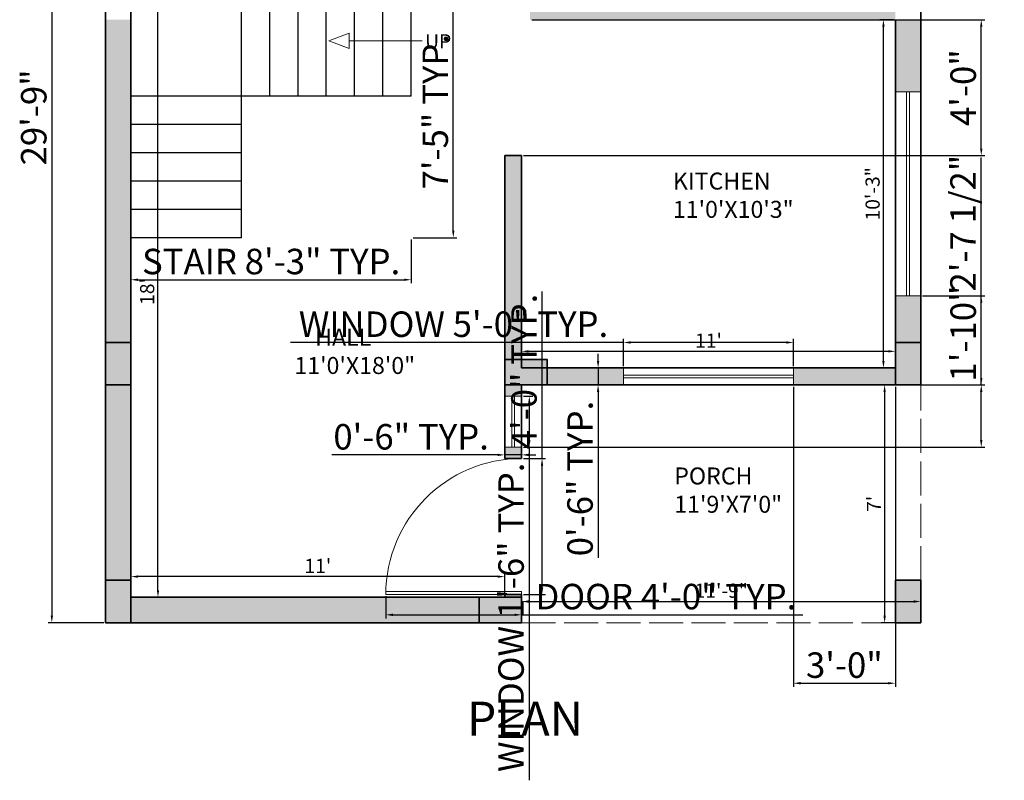
# Model space of a CAD drawing. Units: inches. Extents: x 3148 to 3962, y 1142 to 1671.
# Tile 8 of 9: x 3585 to 3933, y 1142 to 1411. Entities that reach past the tile are written whole.
import ezdxf

# ---------------------------------------------------------------- set-up
doc = ezdxf.new("R2010")
doc.units = ezdxf.units.IN
doc.linetypes.add('ACAD_ISO02W100', pattern=[15, 12, -3])
for name, color, linetype, lineweight in [('A-ANNO-DIMS', 2, 'Continuous', 18), ('A-ANNO-SYMB', 7, 'Continuous', 18), ('A-ANNO-TEXT', 7, 'Continuous', 25), ('A-AREA-IDEN', 7, 'Continuous', 18), ('A-COLS', 1, 'Continuous', 35), ('A-DOOR', 3, 'Continuous', 18), ('A-FLOR-STRS', 7, 'Continuous', 25), ('A-GLAZ', 4, 'Continuous', 18), ('A-ROOF-OVHD', 7, 'ACAD_ISO02W100', 18), ('A-WALL', 7, 'Continuous', 35)]:
    doc.layers.add(name, color=color, linetype=linetype, lineweight=lineweight)
doc.layers.add('A-WALL-PATT', color=252, linetype='Continuous', lineweight=13, true_color=0x939598)
doc.styles.get("Standard").update_dxf_attribs({"font": 'arial.ttf'})
doc.dimstyles.new('ISO-25', dxfattribs={"dimtxt": 9, "dimasz": 2.5, "dimexe": 1.25, "dimexo": 0.625, "dimtad": 1, "dimdec": 1, "dimlunit": 3, "dimtxsty": 'Standard', "dimcen": 2.5, "dimadec": 0, "dimazin": 0, "dimtfac": 1, "dimtdec": 1, "dimtmove": 0, "dimatfit": 3, "dimfxl": 1, "dimarcsym": 0})

# ---------------------------------------------------------------- blocks, each defined once
blk = doc.blocks.new('*D45')
at = {"layer": 'A-ANNO-DIMS', "color": 0, "lineweight": -2, "transparency": 16777216}
for p, q in [((3614.71, 1554.8), (3595.12, 1554.8)), ((3596.37, 1552.3), (3596.37, 1200.3)), ((3614.71, 1197.8), (3595.12, 1197.8))]:
    blk.add_line(p, q, dxfattribs=at)
at = {"layer": 'A-ANNO-DIMS', "color": 0, "transparency": 16777216}
for points in [[(3595.95, 1552.3), (3596.78, 1552.3), (3596.37, 1554.8)], [(3595.95, 1200.3), (3596.78, 1200.3), (3596.37, 1197.8)]]:
    blk.add_solid(points, dxfattribs=at)
at = {"layer": 'Defpoints', "color": 0, "transparency": 16777216}
for p in [(3615.33, 1554.8), (3596.37, 1197.8), (3615.33, 1197.8)]:
    blk.add_point(p, dxfattribs=at)
at = {"layer": 'A-ANNO-DIMS', "color": 0, "transparency": 16777216, "insert": (3591.15, 1376.3), "char_height": 9, "attachment_point": 5, "rotation": 90}
blk.add_mtext('29\'-9"', dxfattribs=at)
blk = doc.blocks.new('*D46')
at = {"layer": 'A-ANNO-DIMS', "color": 0, "lineweight": -2, "transparency": 16777216}
for p, q in [((3624.96, 1422.8), (3635.11, 1422.8)), ((3633.86, 1209.3), (3633.86, 1420.3)), ((3624.96, 1206.8), (3635.11, 1206.8))]:
    blk.add_line(p, q, dxfattribs=at)
at = {"layer": 'A-ANNO-DIMS', "color": 0, "transparency": 16777216}
for points in [[(3633.45, 1420.3), (3634.28, 1420.3), (3633.86, 1422.8)], [(3633.45, 1209.3), (3634.28, 1209.3), (3633.86, 1206.8)]]:
    blk.add_solid(points, dxfattribs=at)
at = {"layer": 'Defpoints', "color": 0, "transparency": 16777216}
for p in [(3624.33, 1422.8), (3633.86, 1422.8), (3624.33, 1206.8)]:
    blk.add_point(p, dxfattribs=at)
at = {"layer": 'A-ANNO-DIMS', "color": 0, "transparency": 16777216, "insert": (3630.69, 1314.8), "char_height": 5, "attachment_point": 5, "rotation": 90}
blk.add_mtext("18'", dxfattribs=at)
blk = doc.blocks.new('*D47')
at = {"layer": 'A-ANNO-DIMS', "color": 0, "lineweight": -2, "transparency": 16777216}
for p, q in [((3624.33, 1207.42), (3624.33, 1215.36)), ((3753.83, 1214.11), (3626.83, 1214.11)), ((3756.33, 1207.42), (3756.33, 1215.36))]:
    blk.add_line(p, q, dxfattribs=at)
at = {"layer": 'A-ANNO-DIMS', "color": 0, "transparency": 16777216}
for points in [[(3626.83, 1214.53), (3626.83, 1213.69), (3624.33, 1214.11)], [(3753.83, 1214.53), (3753.83, 1213.69), (3756.33, 1214.11)]]:
    blk.add_solid(points, dxfattribs=at)
at = {"layer": 'Defpoints', "color": 0, "transparency": 16777216}
for p in [(3624.33, 1214.11), (3624.33, 1206.8), (3756.33, 1206.8)]:
    blk.add_point(p, dxfattribs=at)
at = {"layer": 'A-ANNO-DIMS', "color": 0, "transparency": 16777216, "insert": (3690.33, 1217.24), "char_height": 5, "attachment_point": 5}
blk.add_mtext("11'", dxfattribs=at)
blk = doc.blocks.new('*D48')
at = {"layer": 'A-ANNO-DIMS', "color": 0, "lineweight": -2, "transparency": 16777216}
for p, q in [((3762.33, 1198.42), (3762.33, 1206.55)), ((3764.83, 1205.3), (3900.83, 1205.3)), ((3903.33, 1198.42), (3903.33, 1206.55))]:
    blk.add_line(p, q, dxfattribs=at)
at = {"layer": 'A-ANNO-DIMS', "color": 0, "transparency": 16777216}
for points in [[(3764.83, 1205.72), (3764.83, 1204.88), (3762.33, 1205.3)], [(3900.83, 1205.72), (3900.83, 1204.88), (3903.33, 1205.3)]]:
    blk.add_solid(points, dxfattribs=at)
at = {"layer": 'Defpoints', "color": 0, "transparency": 16777216}
for p in [(3903.33, 1205.3), (3762.33, 1197.8), (3903.33, 1197.8)]:
    blk.add_point(p, dxfattribs=at)
at = {"layer": 'A-ANNO-DIMS', "color": 0, "transparency": 16777216, "insert": (3832.83, 1208.48), "char_height": 5, "attachment_point": 5}
blk.add_mtext('11\'-9"', dxfattribs=at)
blk = doc.blocks.new('*D49')
at = {"layer": 'A-ANNO-DIMS', "color": 0, "lineweight": -2, "transparency": 16777216}
for p, q in [((3902.71, 1281.8), (3889.3, 1281.8)), ((3890.55, 1279.3), (3890.55, 1200.3)), ((3902.71, 1197.8), (3889.3, 1197.8))]:
    blk.add_line(p, q, dxfattribs=at)
at = {"layer": 'A-ANNO-DIMS', "color": 0, "transparency": 16777216}
for points in [[(3890.13, 1279.3), (3890.96, 1279.3), (3890.55, 1281.8)], [(3890.13, 1200.3), (3890.96, 1200.3), (3890.55, 1197.8)]]:
    blk.add_solid(points, dxfattribs=at)
at = {"layer": 'Defpoints', "color": 0, "transparency": 16777216}
for p in [(3903.33, 1281.8), (3890.55, 1197.8), (3903.33, 1197.8)]:
    blk.add_point(p, dxfattribs=at)
at = {"layer": 'A-ANNO-DIMS', "color": 0, "transparency": 16777216, "insert": (3887.42, 1239.8), "char_height": 5, "attachment_point": 5, "rotation": 90}
blk.add_mtext("7'", dxfattribs=at)
blk = doc.blocks.new('*D50')
at = {"layer": 'A-ANNO-DIMS', "color": 0, "lineweight": -2, "transparency": 16777216}
for p, q in [((3762.33, 1291.42), (3762.33, 1294.93)), ((3894.33, 1291.42), (3894.33, 1294.93)), ((3764.83, 1293.68), (3891.83, 1293.68))]:
    blk.add_line(p, q, dxfattribs=at)
at = {"layer": 'A-ANNO-DIMS', "color": 0, "transparency": 16777216}
for points in [[(3764.83, 1294.09), (3764.83, 1293.26), (3762.33, 1293.68)], [(3891.83, 1294.09), (3891.83, 1293.26), (3894.33, 1293.68)]]:
    blk.add_solid(points, dxfattribs=at)
at = {"layer": 'Defpoints', "color": 0, "transparency": 16777216}
for p in [(3762.33, 1290.8), (3894.33, 1293.68), (3894.33, 1290.8)]:
    blk.add_point(p, dxfattribs=at)
at = {"layer": 'A-ANNO-DIMS', "color": 0, "transparency": 16777216, "insert": (3828.33, 1296.81), "char_height": 5, "attachment_point": 5}
blk.add_mtext("11'", dxfattribs=at)
blk = doc.blocks.new('*D51')
at = {"layer": 'A-ANNO-DIMS', "color": 0, "lineweight": -2, "transparency": 16777216}
for p, q in [((3893.71, 1410.8), (3888.88, 1410.8)), ((3890.13, 1290.3), (3890.13, 1408.3)), ((3893.71, 1287.8), (3888.88, 1287.8))]:
    blk.add_line(p, q, dxfattribs=at)
at = {"layer": 'A-ANNO-DIMS', "color": 0, "transparency": 16777216}
for points in [[(3889.71, 1408.3), (3890.55, 1408.3), (3890.13, 1410.8)], [(3889.71, 1290.3), (3890.55, 1290.3), (3890.13, 1287.8)]]:
    blk.add_solid(points, dxfattribs=at)
at = {"layer": 'Defpoints', "color": 0, "transparency": 16777216}
for p in [(3890.13, 1410.8), (3894.33, 1410.8), (3894.33, 1287.8)]:
    blk.add_point(p, dxfattribs=at)
at = {"layer": 'A-ANNO-DIMS', "color": 0, "transparency": 16777216, "insert": (3886.95, 1349.3), "char_height": 5, "attachment_point": 5, "rotation": 90}
blk.add_mtext('10\'-3"', dxfattribs=at)
blk = doc.blocks.new('DOOR-SWING-48')
for p, q in [((-48, 0), (0, 0)), ((-47.99, 1), (0, 1)), ((0, 0), (0, 1))]:
    blk.add_line(p, q)
blk.add_arc((0, 0), 48, 90, 180)
blk = doc.blocks.new('WIN-18')
for p, q in [((0, 18), (6, 18)), ((2.5, 0), (2.5, 18)), ((3.5, 0), (3.5, 18)), ((0, 0), (6, 0))]:
    blk.add_line(p, q)
blk = doc.blocks.new('WIN-60')
for p, q in [((0, 0), (0, 6)), ((60, 3.5), (0, 3.5)), ((60, 0), (60, 6)), ((60, 2.5), (0, 2.5))]:
    blk.add_line(p, q)
blk = doc.blocks.new('WIN-72')
for p, q in [((0, 72), (9, 72)), ((4, 72), (4, 0)), ((5, 72), (5, 0)), ((0, 0), (9, 0))]:
    blk.add_line(p, q)
blk = doc.blocks.new('STAIR-QUARTER-TURN')
for p, q in [((39, 0), (39, 89)), ((49, 50), (49, 89)), ((59, 50), (59, 89)), ((69, 50), (69, 89)), ((79, 50), (79, 89)), ((89, 50), (89, 89)), ((99, 50), (99, 89)), ((99, 50), (0, 50)), ((39, 40), (0, 40)), ((39, 30), (0, 30)), ((39, 20), (0, 20)), ((39, 10), (0, 10)), ((39, 0), (0, 0))]:
    blk.add_line(p, q)
blk = doc.blocks.new('COL-9X15')
h = blk.add_hatch(color=256)
h.dxf.hatch_style = 1
h.paths.add_polyline_path([(9, 15), (0, 15), (0, 0), (9, 0)])
blk.add_lwpolyline([(9, 0), (9, 15), (0, 15), (0, 0)], close=True)
blk = doc.blocks.new('STAIR-UP-ARROW')
blk.add_line((32.89, 2.71), (7.09, 2.71))
blk.add_lwpolyline([(0, 2.71), (7.09, 0), (7.09, 5.42)], close=True)
blk.add_text('UP', height=5).set_placement((33.98, 0.05))
blk = doc.blocks.new('*D76')
at = {"layer": 'A-ANNO-DIMS', "color": 0, "lineweight": -2, "transparency": 16777216}
for p, q in [((3762.96, 1277.8), (3766.28, 1277.8)), ((3765.03, 1275.3), (3765.03, 1262.3)), ((3762.96, 1259.8), (3766.28, 1259.8)), ((3765.03, 1259.8), (3765.03, 1142.16))]:
    blk.add_line(p, q, dxfattribs=at)
at = {"layer": 'A-ANNO-DIMS', "color": 0, "transparency": 16777216}
for points in [[(3764.61, 1275.3), (3765.45, 1275.3), (3765.03, 1277.8)], [(3764.61, 1262.3), (3765.45, 1262.3), (3765.03, 1259.8)]]:
    blk.add_solid(points, dxfattribs=at)
at = {"layer": 'Defpoints', "color": 0, "transparency": 16777216}
for p in [(3762.33, 1277.8), (3762.33, 1259.8), (3765.03, 1259.8)]:
    blk.add_point(p, dxfattribs=at)
at = {"layer": 'A-ANNO-DIMS', "color": 0, "transparency": 16777216, "insert": (3759.75, 1199.73), "char_height": 9, "attachment_point": 5, "rotation": 90}
blk.add_mtext('WINDOW 1\'-6" TYP.', dxfattribs=at)
blk = doc.blocks.new('*D77')
at = {"layer": 'A-ANNO-DIMS', "color": 0, "lineweight": -2, "transparency": 16777216}
for p, q in [((3756.33, 1259.17), (3756.33, 1255.85)), ((3762.33, 1259.17), (3762.33, 1255.85)), ((3753.83, 1257.1), (3695.22, 1257.1)), ((3762.33, 1257.1), (3756.33, 1257.1)), ((3764.83, 1257.1), (3767.33, 1257.1))]:
    blk.add_line(p, q, dxfattribs=at)
at = {"layer": 'A-ANNO-DIMS', "color": 0, "transparency": 16777216}
for points in [[(3753.83, 1257.52), (3753.83, 1256.68), (3756.33, 1257.1)], [(3764.83, 1257.52), (3764.83, 1256.68), (3762.33, 1257.1)]]:
    blk.add_solid(points, dxfattribs=at)
at = {"layer": 'Defpoints', "color": 0, "transparency": 16777216}
for p in [(3756.33, 1259.8), (3762.33, 1259.8), (3756.33, 1257.1)]:
    blk.add_point(p, dxfattribs=at)
at = {"layer": 'A-ANNO-DIMS', "color": 0, "transparency": 16777216, "insert": (3723.28, 1262.32), "char_height": 9, "attachment_point": 5}
blk.add_mtext('0\'-6" TYP.', dxfattribs=at)
blk = doc.blocks.new('*D78')
at = {"layer": 'A-ANNO-DIMS', "color": 0, "lineweight": -2, "transparency": 16777216}
for p, q in [((3798.33, 1288.42), (3798.33, 1298.05)), ((3858.33, 1288.42), (3858.33, 1298.05)), ((3798.33, 1296.8), (3680.69, 1296.8)), ((3855.83, 1296.8), (3800.83, 1296.8))]:
    blk.add_line(p, q, dxfattribs=at)
at = {"layer": 'A-ANNO-DIMS', "color": 0, "transparency": 16777216}
for points in [[(3800.83, 1297.22), (3800.83, 1296.38), (3798.33, 1296.8)], [(3855.83, 1297.22), (3855.83, 1296.38), (3858.33, 1296.8)]]:
    blk.add_solid(points, dxfattribs=at)
at = {"layer": 'Defpoints', "color": 0, "transparency": 16777216}
for p in [(3798.33, 1296.8), (3798.33, 1287.8), (3858.33, 1287.8)]:
    blk.add_point(p, dxfattribs=at)
at = {"layer": 'A-ANNO-DIMS', "color": 0, "transparency": 16777216, "insert": (3738.26, 1302.08), "char_height": 9, "attachment_point": 5}
blk.add_mtext('WINDOW 5\'-0" TYP.', dxfattribs=at)
blk = doc.blocks.new('*D79')
at = {"layer": 'A-ANNO-DIMS', "color": 0, "lineweight": -2, "transparency": 16777216}
for p, q in [((3789.33, 1290.3), (3789.33, 1292.8)), ((3797.71, 1287.8), (3788.08, 1287.8)), ((3789.33, 1287.8), (3789.33, 1281.8)), ((3797.71, 1281.8), (3788.08, 1281.8)), ((3789.33, 1279.3), (3789.33, 1220.69))]:
    blk.add_line(p, q, dxfattribs=at)
at = {"layer": 'A-ANNO-DIMS', "color": 0, "transparency": 16777216}
for points in [[(3788.91, 1290.3), (3789.75, 1290.3), (3789.33, 1287.8)], [(3788.91, 1279.3), (3789.75, 1279.3), (3789.33, 1281.8)]]:
    blk.add_solid(points, dxfattribs=at)
at = {"layer": 'Defpoints', "color": 0, "transparency": 16777216}
for p in [(3798.33, 1287.8), (3789.33, 1281.8), (3798.33, 1281.8)]:
    blk.add_point(p, dxfattribs=at)
at = {"layer": 'A-ANNO-DIMS', "color": 0, "transparency": 16777216, "insert": (3784.11, 1248.74), "char_height": 9, "attachment_point": 5, "rotation": 90}
blk.add_mtext('0\'-6" TYP.', dxfattribs=at)
blk = doc.blocks.new('*D84')
at = {"layer": 'A-ANNO-DIMS', "color": 0, "lineweight": -2, "transparency": 16777216}
for p, q in [((3714.33, 1207.17), (3714.33, 1199.35)), ((3762.33, 1207.17), (3762.33, 1199.35)), ((3716.83, 1200.6), (3759.83, 1200.6)), ((3762.33, 1200.6), (3861.7, 1200.6))]:
    blk.add_line(p, q, dxfattribs=at)
at = {"layer": 'A-ANNO-DIMS', "color": 0, "transparency": 16777216}
for points in [[(3716.83, 1201.02), (3716.83, 1200.18), (3714.33, 1200.6)], [(3759.83, 1201.02), (3759.83, 1200.18), (3762.33, 1200.6)]]:
    blk.add_solid(points, dxfattribs=at)
at = {"layer": 'Defpoints', "color": 0, "transparency": 16777216}
for p in [(3714.33, 1207.8), (3762.33, 1207.8), (3762.33, 1200.6)]:
    blk.add_point(p, dxfattribs=at)
at = {"layer": 'A-ANNO-DIMS', "color": 0, "transparency": 16777216, "insert": (3813.27, 1205.88), "char_height": 9, "attachment_point": 5}
blk.add_mtext('DOOR 4\'-0" TYP.', dxfattribs=at)
blk = doc.blocks.new('*D85')
at = {"layer": 'A-ANNO-DIMS', "color": 0, "lineweight": -2, "transparency": 16777216}
for p, q in [((3769.53, 1255.8), (3769.53, 1314.77)), ((3762.96, 1255.8), (3770.78, 1255.8)), ((3769.53, 1210.3), (3769.53, 1253.3)), ((3762.96, 1207.8), (3770.78, 1207.8))]:
    blk.add_line(p, q, dxfattribs=at)
at = {"layer": 'A-ANNO-DIMS', "color": 0, "transparency": 16777216}
for points in [[(3769.11, 1253.3), (3769.95, 1253.3), (3769.53, 1255.8)], [(3769.11, 1210.3), (3769.95, 1210.3), (3769.53, 1207.8)]]:
    blk.add_solid(points, dxfattribs=at)
at = {"layer": 'Defpoints', "color": 0, "transparency": 16777216}
for p in [(3762.33, 1255.8), (3769.53, 1255.8), (3762.33, 1207.8)]:
    blk.add_point(p, dxfattribs=at)
at = {"layer": 'A-ANNO-DIMS', "color": 0, "transparency": 16777216, "insert": (3764.31, 1286.54), "char_height": 9, "attachment_point": 5, "rotation": 90}
blk.add_mtext('4\'-0" TYP.', dxfattribs=at)
blk = doc.blocks.new('*D86')
at = {"layer": 'A-ANNO-DIMS', "color": 0, "lineweight": -2, "transparency": 16777216}
for p, q in [((3624.33, 1333.17), (3624.33, 1317.7)), ((3723.33, 1333.17), (3723.33, 1317.7)), ((3626.83, 1318.95), (3720.83, 1318.95))]:
    blk.add_line(p, q, dxfattribs=at)
at = {"layer": 'A-ANNO-DIMS', "color": 0, "transparency": 16777216}
for points in [[(3626.83, 1319.37), (3626.83, 1318.53), (3624.33, 1318.95)], [(3720.83, 1319.37), (3720.83, 1318.53), (3723.33, 1318.95)]]:
    blk.add_solid(points, dxfattribs=at)
at = {"layer": 'Defpoints', "color": 0, "transparency": 16777216}
for p in [(3624.33, 1333.8), (3723.33, 1333.8), (3723.33, 1318.95)]:
    blk.add_point(p, dxfattribs=at)
at = {"layer": 'A-ANNO-DIMS', "color": 0, "transparency": 16777216, "insert": (3673.83, 1324.23), "char_height": 9, "attachment_point": 5}
blk.add_mtext('STAIR 8\'-3" TYP.', dxfattribs=at)
blk = doc.blocks.new('*D87')
at = {"layer": 'A-ANNO-DIMS', "color": 0, "lineweight": -2, "transparency": 16777216}
for p, q in [((3723.96, 1422.8), (3739.43, 1422.8)), ((3738.18, 1336.3), (3738.18, 1420.3)), ((3723.96, 1333.8), (3739.43, 1333.8))]:
    blk.add_line(p, q, dxfattribs=at)
at = {"layer": 'A-ANNO-DIMS', "color": 0, "transparency": 16777216}
for points in [[(3737.76, 1420.3), (3738.6, 1420.3), (3738.18, 1422.8)], [(3737.76, 1336.3), (3738.6, 1336.3), (3738.18, 1333.8)]]:
    blk.add_solid(points, dxfattribs=at)
at = {"layer": 'Defpoints', "color": 0, "transparency": 16777216}
for p in [(3723.33, 1422.8), (3738.18, 1422.8), (3723.33, 1333.8)]:
    blk.add_point(p, dxfattribs=at)
at = {"layer": 'A-ANNO-DIMS', "color": 0, "transparency": 16777216, "insert": (3732.98, 1378.3), "char_height": 9, "attachment_point": 5, "rotation": 90}
blk.add_mtext('7\'-5" TYP.', dxfattribs=at)
blk = doc.blocks.new('*D113')
at = {"layer": 'A-ANNO-DIMS', "color": 0, "lineweight": -2, "transparency": 16777216}
for p, q in [((3765.96, 1410.8), (3925.93, 1410.8)), ((3924.68, 1365.3), (3924.68, 1408.3)), ((3762.96, 1362.8), (3925.93, 1362.8))]:
    blk.add_line(p, q, dxfattribs=at)
at = {"layer": 'A-ANNO-DIMS', "color": 0, "transparency": 16777216}
for points in [[(3924.26, 1408.3), (3925.1, 1408.3), (3924.68, 1410.8)], [(3924.26, 1365.3), (3925.1, 1365.3), (3924.68, 1362.8)]]:
    blk.add_solid(points, dxfattribs=at)
at = {"layer": 'Defpoints', "color": 0, "transparency": 16777216}
for p in [(3765.33, 1410.8), (3924.68, 1410.8), (3762.33, 1362.8)]:
    blk.add_point(p, dxfattribs=at)
at = {"layer": 'A-ANNO-DIMS', "color": 0, "transparency": 16777216, "insert": (3919.46, 1386.8), "char_height": 9, "attachment_point": 5, "rotation": 90}
blk.add_mtext('4\'-0"', dxfattribs=at)
blk = doc.blocks.new('*D115')
at = {"layer": 'A-ANNO-DIMS', "color": 0, "lineweight": -2, "transparency": 16777216}
for p, q in [((3924.68, 1313.3), (3924.68, 1362.1)), ((3903.96, 1313.3), (3925.93, 1313.3)), ((3924.68, 1284.3), (3924.68, 1310.8)), ((3903.96, 1281.8), (3925.93, 1281.8))]:
    blk.add_line(p, q, dxfattribs=at)
at = {"layer": 'A-ANNO-DIMS', "color": 0, "transparency": 16777216}
for points in [[(3924.26, 1310.8), (3925.1, 1310.8), (3924.68, 1313.3)], [(3924.26, 1284.3), (3925.1, 1284.3), (3924.68, 1281.8)]]:
    blk.add_solid(points, dxfattribs=at)
at = {"layer": 'Defpoints', "color": 0, "transparency": 16777216}
for p in [(3903.33, 1313.3), (3924.68, 1313.3), (3903.33, 1281.8)]:
    blk.add_point(p, dxfattribs=at)
at = {"layer": 'A-ANNO-DIMS', "color": 0, "transparency": 16777216, "insert": (3919.4, 1338.95), "char_height": 9, "attachment_point": 5, "rotation": 90}
blk.add_mtext('2\'-7 1/2"', dxfattribs=at)
blk = doc.blocks.new('*D116')
at = {"layer": 'A-ANNO-DIMS', "color": 0, "lineweight": -2, "transparency": 16777216}
for p, q in [((3858.33, 1281.17), (3858.33, 1175.2)), ((3894.33, 1281.17), (3894.33, 1175.2)), ((3860.83, 1176.45), (3891.83, 1176.45))]:
    blk.add_line(p, q, dxfattribs=at)
at = {"layer": 'A-ANNO-DIMS', "color": 0, "transparency": 16777216}
for points in [[(3860.83, 1176.87), (3860.83, 1176.03), (3858.33, 1176.45)], [(3891.83, 1176.87), (3891.83, 1176.03), (3894.33, 1176.45)]]:
    blk.add_solid(points, dxfattribs=at)
at = {"layer": 'Defpoints', "color": 0, "transparency": 16777216}
for p in [(3858.33, 1281.8), (3894.33, 1281.8), (3894.33, 1176.45)]:
    blk.add_point(p, dxfattribs=at)
at = {"layer": 'A-ANNO-DIMS', "color": 0, "transparency": 16777216, "insert": (3876.33, 1181.67), "char_height": 9, "attachment_point": 5}
blk.add_mtext('3\'-0"', dxfattribs=at)
blk = doc.blocks.new('*D120')
at = {"layer": 'A-ANNO-DIMS', "color": 0, "lineweight": -2, "transparency": 16777216}
for p, q in [((3924.68, 1281.8), (3924.68, 1315.62)), ((3762.96, 1281.8), (3925.93, 1281.8)), ((3924.68, 1262.3), (3924.68, 1279.3)), ((3762.96, 1259.8), (3925.93, 1259.8))]:
    blk.add_line(p, q, dxfattribs=at)
at = {"layer": 'A-ANNO-DIMS', "color": 0, "transparency": 16777216}
for points in [[(3924.26, 1279.3), (3925.1, 1279.3), (3924.68, 1281.8)], [(3924.26, 1262.3), (3925.1, 1262.3), (3924.68, 1259.8)]]:
    blk.add_solid(points, dxfattribs=at)
at = {"layer": 'Defpoints', "color": 0, "transparency": 16777216}
for p in [(3762.33, 1281.8), (3924.68, 1281.8), (3762.33, 1259.8)]:
    blk.add_point(p, dxfattribs=at)
at = {"layer": 'A-ANNO-DIMS', "color": 0, "transparency": 16777216, "insert": (3919.46, 1299.96), "char_height": 9, "attachment_point": 5, "rotation": 90}
blk.add_mtext('1\'-10"', dxfattribs=at)

msp = doc.modelspace()

# ---------------------------------------------------------------- hatches: boundary and pattern name
at = {"layer": 'A-WALL-PATT'}
h = msp.add_hatch(color=256, dxfattribs=at)
h.dxf.hatch_style = 1
h.paths.add_polyline_path([(3624.33, 1410.8), (3615.33, 1410.8), (3615.33, 1296.8), (3624.33, 1296.8), (3624.33, 1300.86)])
h.paths.add_polyline_path([(3624.33, 1281.8), (3615.33, 1281.8), (3615.33, 1212.8), (3624.33, 1212.8)])
h.paths.add_polyline_path([(3747.33, 1206.8), (3624.33, 1206.8), (3624.33, 1197.8), (3747.33, 1197.8)])
h.paths.add_polyline_path([(3762.33, 1362.8), (3756.33, 1362.8), (3756.33, 1290.8), (3762.33, 1290.8)])
h.paths.add_polyline_path([(3762.33, 1207.8), (3756.33, 1207.8), (3756.33, 1206.8), (3762.33, 1206.8)])
h.paths.add_polyline_path([(3762.33, 1259.8), (3756.33, 1259.8), (3756.33, 1255.8), (3762.33, 1255.8)])
h.paths.add_polyline_path([(3762.33, 1281.8), (3756.33, 1281.8), (3756.33, 1277.8), (3762.33, 1277.8)])
h.paths.add_polyline_path([(3798.33, 1287.8), (3771.33, 1287.8), (3771.33, 1281.8), (3798.33, 1281.8)])
h.paths.add_polyline_path([(3894.33, 1287.8), (3866.33, 1287.8), (3858.33, 1287.8), (3858.33, 1281.8), (3894.33, 1281.8)])
h.paths.add_polyline_path([(3903.33, 1313.3), (3894.33, 1313.3), (3894.33, 1296.8), (3903.33, 1296.8)])
h.paths.add_polyline_path([(3903.33, 1410.8), (3894.33, 1410.8), (3894.33, 1385.3), (3903.33, 1385.3)])
h.paths.add_polyline_path([(3894.33, 1416.8), (3765.33, 1416.8), (3765.33, 1410.8), (3894.33, 1410.8)])
h.paths.add_polyline_path([(3903.33, 1445.3), (3894.33, 1445.3), (3894.33, 1425.8), (3903.33, 1425.8)])
h.paths.add_polyline_path([(3762.33, 1426.3), (3756.33, 1426.3), (3756.33, 1425.8), (3762.33, 1425.8)])
h.paths.add_polyline_path([(3725.33, 1428.8), (3674.83, 1428.8), (3674.83, 1430.3), (3672.33, 1430.3), (3672.33, 1428.8), (3624.33, 1428.8), (3624.33, 1512.8), (3636.33, 1512.8), (3636.33, 1518.8), (3624.33, 1518.8), (3624.33, 1539.8), (3615.33, 1539.8), (3615.33, 1425.8), (3624.33, 1425.8), (3624.33, 1422.8), (3725.33, 1422.8)])
h.paths.add_polyline_path([(3686.83, 1518.8), (3660.33, 1518.8), (3660.33, 1512.8), (3672.33, 1512.8), (3672.33, 1461.3), (3674.83, 1461.3), (3674.83, 1462.3), (3676.83, 1462.3), (3676.83, 1464.8), (3674.83, 1464.8), (3674.83, 1512.8), (3686.83, 1512.8)], flags=17)
h.paths.add_polyline_path([(3728.83, 1518.8), (3710.83, 1518.8), (3710.83, 1512.8), (3722.83, 1512.8), (3722.83, 1464.8), (3707.83, 1464.8), (3707.83, 1462.3), (3725.33, 1462.3), (3725.33, 1512.8), (3728.83, 1512.8)])
h.paths.add_polyline_path([(3762.33, 1539.8), (3756.33, 1539.8), (3756.33, 1518.8), (3752.83, 1518.8), (3752.83, 1512.8), (3756.33, 1512.8), (3756.33, 1462.3), (3762.33, 1462.3)])
h.paths.add_polyline_path([(3756.33, 1554.8), (3624.33, 1554.8), (3624.33, 1545.8), (3756.33, 1545.8)])
h.paths.add_polyline_path([(3894.33, 1554.8), (3765.33, 1554.8), (3765.33, 1545.8), (3784.23, 1545.8), (3894.33, 1545.8)])
h.paths.add_polyline_path([(3903.33, 1539.8), (3894.33, 1539.8), (3894.33, 1517.3), (3903.33, 1517.3)])

# ---------------------------------------------------------------- linework, layer by layer
at = {"layer": 'A-ROOF-OVHD'}
for p, q in [((3903.33, 1197.8), (3903.33, 1281.8)), ((3762.33, 1197.8), (3903.33, 1197.8))]:
    msp.add_line(p, q, dxfattribs=at)
at = {"layer": 'A-WALL'}
for p, q in [((3615.33, 1197.8), (3615.33, 1554.8)), ((3903.33, 1554.8), (3903.33, 1281.8)), ((3624.33, 1206.8), (3624.33, 1422.8)), ((3894.33, 1410.8), (3894.33, 1287.8)), ((3756.33, 1362.8), (3756.33, 1255.8)), ((3762.33, 1362.8), (3756.33, 1362.8)), ((3762.33, 1362.8), (3762.33, 1287.8)), ((3762.33, 1287.8), (3894.33, 1287.8)), ((3762.33, 1281.8), (3894.33, 1281.8)), ((3762.33, 1281.8), (3762.33, 1255.8)), ((3762.33, 1255.8), (3756.33, 1255.8)), ((3756.33, 1207.8), (3756.33, 1206.8)), ((3762.33, 1207.8), (3756.33, 1207.8)), ((3762.33, 1207.8), (3762.33, 1206.8)), ((3762.33, 1206.8), (3624.33, 1206.8)), ((3762.33, 1206.8), (3762.33, 1197.8)), ((3762.33, 1197.8), (3615.33, 1197.8))]:
    msp.add_line(p, q, dxfattribs=at)

# ---------------------------------------------------------------- block references
at = {"layer": 'A-ANNO-SYMB'}
msp.add_blockref('STAIR-UP-ARROW', (3694.26, 1400.59), dxfattribs=at)
at = {"layer": 'A-COLS'}
for p in [(3615.33, 1281.8), (3894.33, 1281.8), (3615.33, 1197.8), (3894.33, 1197.8)]:
    msp.add_blockref('COL-9X15', p, dxfattribs=at)
for p, rotation in [((3756.33, 1290.8), 270.0000000000012), ((3747.33, 1206.8), 270.0000000000023)]:
    msp.add_blockref('COL-9X15', p, dxfattribs=dict(at, rotation=rotation))
at = {"layer": 'A-DOOR'}
msp.add_blockref('DOOR-SWING-48', (3762.33, 1207.8), dxfattribs=at)
at = {"layer": 'A-FLOR-STRS'}
msp.add_blockref('STAIR-QUARTER-TURN', (3624.33, 1333.8), dxfattribs=at)
at = {"layer": 'A-GLAZ'}
msp.add_blockref('WIN-72', (3894.33, 1313.3), dxfattribs=at)
at = {"layer": 'A-GLAZ', "rotation": 180}
for name, p in [('WIN-60', (3858.33, 1287.8)), ('WIN-18', (3762.33, 1277.8))]:
    msp.add_blockref(name, p, dxfattribs=at)

# ---------------------------------------------------------------- texts
at = {"layer": 'A-ANNO-TEXT', "insert": (3743.01, 1169.94), "char_height": 12, "attachment_point": 1}
msp.add_mtext_dynamic_manual_height_columns('PLAN', width=77.9518, gutter_width=12.5, heights=[0], dxfattribs=at)
at = {"layer": 'A-AREA-IDEN', "char_height": 6, "attachment_point": 1}
for s, insert in [('KITCHEN\\P11\'0\'X10\'3"', (3815.75, 1356.81)), ('    HALL\\P11\'0\'X18\'0"', (3682.05, 1301.67)), ('PORCH\\P11\'9\'X7\'0"', (3816.23, 1252.65))]:
    msp.add_mtext_dynamic_manual_height_columns(s, width=77.9518, gutter_width=12.5, heights=[0], dxfattribs=dict(at, insert=insert))

# ---------------------------------------------------------------- dimensions: what is measured, and where the dimension line sits
at = {"layer": 'A-ANNO-DIMS'}
for base, p1, p2, override, picture, middle in [((3596.37, 1197.8), (3615.33, 1554.8), (3615.33, 1197.8), {"dimclrd": 0, "dimclre": 0, "dimclrt": 0}, '*D45', (3591.15, 1376.3)), ((3633.86, 1422.8), (3624.33, 1206.8), (3624.33, 1422.8), {"dimtxt": 5, "dimclrd": 0, "dimclre": 0, "dimclrt": 0}, '*D46', (3630.69, 1314.8)), ((3924.68, 1410.8), (3762.33, 1362.8), (3765.33, 1410.8), {"dimdec": 1, "dimlfac": 1, "dimrnd": 0, "dimzin": 1, "dimdsep": 46, "dimlunit": 4, "dimfrac": 2}, '*D113', (3919.46, 1386.8)), ((3890.13, 1410.8), (3894.33, 1287.8), (3894.33, 1410.8), {"dimtxt": 5, "dimclrd": 0, "dimclre": 0, "dimclrt": 0}, '*D51', (3886.95, 1349.3)), ((3924.68, 1313.3), (3903.33, 1281.8), (3903.33, 1313.3), {"dimdec": 1, "dimlfac": 1, "dimrnd": 0, "dimzin": 1, "dimdsep": 46, "dimlunit": 4, "dimfrac": 2}, '*D115', (3919.4, 1338.95)), ((3924.68, 1281.8), (3762.33, 1259.8), (3762.33, 1281.8), {"dimdec": 1, "dimlfac": 1, "dimrnd": 0, "dimzin": 1, "dimdsep": 46, "dimlunit": 4, "dimfrac": 2}, '*D120', (3919.46, 1299.96)), ((3890.55, 1197.8), (3903.33, 1281.8), (3903.33, 1197.8), {"dimtxt": 5, "dimclrd": 0, "dimclre": 0, "dimclrt": 0}, '*D49', (3887.42, 1239.8))]:
    dim = msp.add_linear_dim(base=base, p1=p1, p2=p2, angle=90, dimstyle='ISO-25', override=override, dxfattribs=at)
    dim.commit()
    dim.dimension.update_dxf_attribs({"geometry": picture, "text_midpoint": middle})
for base, p1, p2, angle, text, picture, middle in [((3738.18, 1422.8), (3723.33, 1333.8), (3723.33, 1422.8), 90, '<> TYP.', '*D87', (3732.98, 1378.3)), ((3798.33, 1296.8), (3858.33, 1287.8), (3798.33, 1287.8), 180, 'WINDOW <> TYP.', '*D78', (3738.26, 1302.08)), ((3769.53, 1255.8), (3762.33, 1207.8), (3762.33, 1255.8), 90, '<> TYP.', '*D85', (3764.31, 1286.54)), ((3789.33, 1281.8), (3798.33, 1287.8), (3798.33, 1281.8), 270, '<> TYP.', '*D79', (3784.11, 1248.74)), ((3765.03, 1259.8), (3762.33, 1277.8), (3762.33, 1259.8), 270, 'WINDOW <> TYP.', '*D76', (3759.75, 1199.73)), ((3756.33, 1257.1), (3762.33, 1259.8), (3756.33, 1259.8), 180, '<> TYP.', '*D77', (3723.28, 1262.32))]:
    dim = msp.add_linear_dim(base=base, p1=p1, p2=p2, angle=angle, text=text, dimstyle='ISO-25', override={"dimdec": 1, "dimlfac": 1, "dimrnd": 0, "dimzin": 1, "dimdsep": 46, "dimlunit": 4, "dimfrac": 2}, dxfattribs=at)
    dim.commit()
    dim.dimension.update_dxf_attribs({"geometry": picture, "text_midpoint": middle})
for base, p1, p2, text, picture, middle in [((3723.33, 1318.95), (3624.33, 1333.8), (3723.33, 1333.8), 'STAIR <> TYP.', '*D86', (3673.83, 1324.23)), ((3762.33, 1200.6), (3714.33, 1207.8), (3762.33, 1207.8), 'DOOR <> TYP.', '*D84', (3813.27, 1205.88))]:
    dim = msp.add_linear_dim(base=base, p1=p1, p2=p2, text=text, dimstyle='ISO-25', override={"dimdec": 1, "dimlfac": 1, "dimrnd": 0, "dimzin": 1, "dimdsep": 46, "dimlunit": 4, "dimfrac": 2}, dxfattribs=at)
    dim.commit()
    dim.dimension.update_dxf_attribs({"geometry": picture, "text_midpoint": middle})
for base, p1, p2, override, picture, middle in [((3894.33, 1293.68), (3762.33, 1290.8), (3894.33, 1290.8), {"dimtxt": 5, "dimclrd": 0, "dimclre": 0, "dimclrt": 0}, '*D50', (3828.33, 1296.81)), ((3894.33, 1176.45), (3858.33, 1281.8), (3894.33, 1281.8), {"dimdec": 1, "dimlfac": 1, "dimrnd": 0, "dimzin": 1, "dimdsep": 46, "dimlunit": 4, "dimfrac": 2}, '*D116', (3876.33, 1181.67)), ((3624.33, 1214.11), (3756.33, 1206.8), (3624.33, 1206.8), {"dimtxt": 5, "dimclrd": 0, "dimclre": 0, "dimclrt": 0}, '*D47', (3690.33, 1217.24)), ((3903.33, 1205.3), (3762.33, 1197.8), (3903.33, 1197.8), {"dimtxt": 5, "dimclrd": 0, "dimclre": 0, "dimclrt": 0}, '*D48', (3832.83, 1208.48))]:
    dim = msp.add_linear_dim(base=base, p1=p1, p2=p2, dimstyle='ISO-25', override=override, dxfattribs=at)
    dim.commit()
    dim.dimension.update_dxf_attribs({"geometry": picture, "text_midpoint": middle})

doc.saveas('drawing.dxf')
